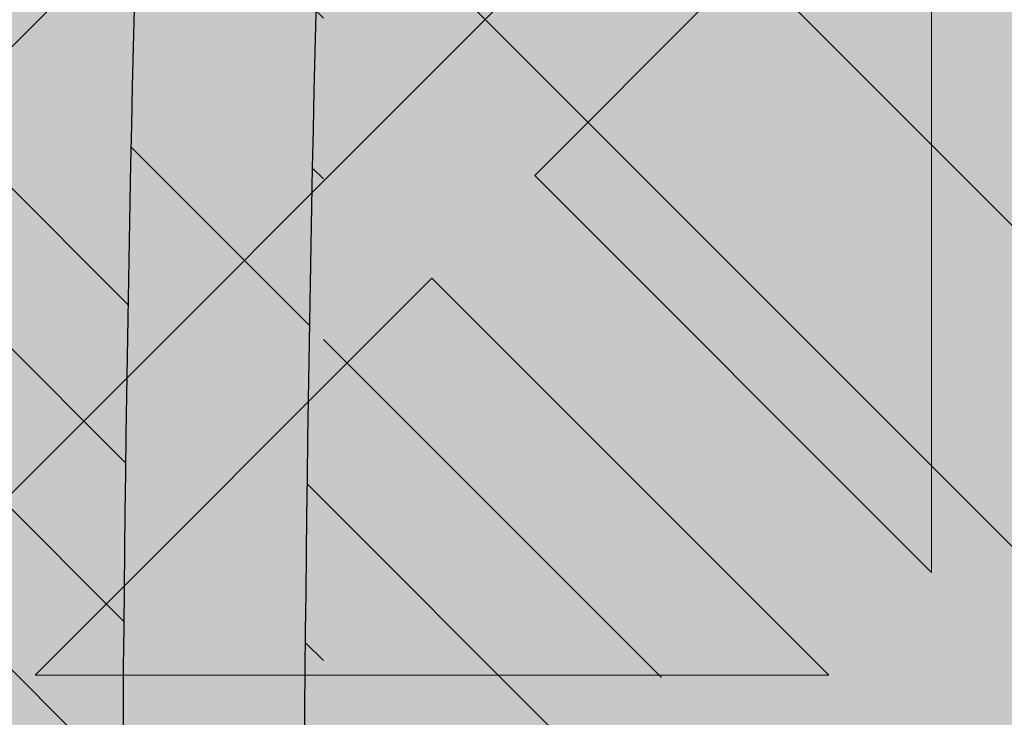
# Model space of a CAD drawing. Units: inches. Extents: x 844 to 2234, y 346 to 1084.
# Tile 80 of 93: x 2002.13 to 2003.858, y 703.938 to 705.162. Entities that reach past the tile are written whole.
import ezdxf

# ---------------------------------------------------------------- set-up
doc = ezdxf.new("R2010")
doc.units = ezdxf.units.IN
doc.header["$MEASUREMENT"] = 0
for name, color, linetype, lineweight in [('A-ANNO-DIMS', 2, 'Continuous', 18), ('furniture', 8, 'Continuous', 18), ('RA-AP-01$0$INT', 35, 'Continuous', 5)]:
    doc.layers.add(name, color=color, linetype=linetype, lineweight=lineweight)
doc.layers.add('RA-AP-01$0$FURN', color=3, linetype='Continuous')
doc.layers.add('RA-AP-01$0$WOOD', color=64, linetype='Continuous')
doc.styles.get("Standard").update_dxf_attribs({"font": 'arial.ttf'})
doc.dimstyles.get("Standard").update_dxf_attribs({"dimtxt": 6, "dimasz": 3, "dimexe": 0.18, "dimexo": 0.0625, "dimgap": 0.09, "dimtad": 0, "dimtih": 1, "dimtoh": 1, "dimdec": 1, "dimzin": 0, "dimdsep": 46, "dimlunit": 3, "dimtxsty": 'Standard', "dimblk": 'ARCHTICK', "dimcen": 0.09, "dimadec": 0, "dimazin": 0, "dimtfac": 1, "dimtdec": 1, "dimtofl": 0, "dimtmove": 0, "dimatfit": 3, "dimfxl": 1, "dimtolj": 1, "dimtzin": 0, "dimarcsym": 0})

# ---------------------------------------------------------------- blocks, each defined once
blk = doc.blocks.new('A$C18D01794')
at = {"layer": 'RA-AP-01$0$INT'}
h = blk.add_hatch(color=256, dxfattribs=at)
h.paths.add_polyline_path([(4.585917135068448, -7.856712009587804), (4.614201406330596, -7.856712009587056), (4.668846067270487, -7.802067348644738), (4.723490728212344, -7.856712009584164), (4.771774999457151, -7.856712009582887), (4.826419660396886, -7.80206734864072), (4.862780050090322, -7.838427738332541), (4.844495778842715, -7.856712009580965), (4.862780050090411, -7.856712009580482), (4.905206456960182, -7.814285602707865), (4.947632863832445, -7.856712009578238), (4.965917135079675, -7.856712009577755), (4.947632863831759, -7.838427738330656), (4.983993253523576, -7.802067348637219), (5.038637914464627, -7.856712009575829), (5.08692218571208, -7.856712009574554), (5.141566846649976, -7.802067348634224), (5.196211507589851, -7.856712009571666), (5.224495778822615, -7.856712009570916), (4.905206456953975, -7.537422687702283)])
h.paths.add_polyline_path([(4.895206456956031, -7.575706958950402), (4.895206456958921, -7.684996280828174), (4.840561796018589, -7.630351619890275)], flags=16)
h.paths.add_polyline_path([(4.915206456955638, -7.575706958949956), (4.969851117895509, -7.630351619887399), (4.915206456957609, -7.684996280827732)], flags=16)
h.paths.add_polyline_path([(4.826419660395175, -7.644493755514321), (4.881064321335613, -7.699138416452331), (4.771774999456703, -7.69913841645522)], flags=16)
h.paths.add_polyline_path([(4.983993253519558, -7.644493755510815), (5.038637914460456, -7.699138416449285), (4.929348592581548, -7.69913841645126)], flags=16)
h.paths.add_polyline_path([(4.881064321336025, -7.719138416452334), (4.826419660397532, -7.773783077393256), (4.771774999457062, -7.719138416455217)], flags=16)
h.paths.add_polyline_path([(4.929348592582019, -7.71913841645126), (5.038637914460982, -7.719138416449284), (4.983993253522945, -7.773783077389749)], flags=16)
h.paths.add_polyline_path([(4.895206456960191, -7.733280552075633), (4.895206456962115, -7.806001331460164), (4.876922185715016, -7.824285602708492), (4.840561796021581, -7.787925213016675)], flags=16)
h.paths.add_polyline_path([(4.915206456958487, -7.733280552075187), (4.969851117899527, -7.787925213013798), (4.933490728206909, -7.824285602708034), (4.9152064569598, -7.806001331461736)], flags=16)
h.paths.add_polyline_path([(4.757632863832376, -7.733280552079264), (4.812277524772842, -7.787925213017304), (4.757632863834348, -7.842569873958233)], flags=16)
h.paths.add_polyline_path([(4.737632863832376, -7.73328055207979), (4.737632863834348, -7.842569873958701), (4.682988202893906, -7.787925213020692)], flags=16)
h.paths.add_polyline_path([(5.05278005008503, -7.733280552072701), (5.052780050087917, -7.842569873951664), (4.998135389146995, -7.787925213013169)], flags=16)
h.paths.add_polyline_path([(5.072780050085024, -7.733280552072333), (5.127424711025931, -7.787925213010806), (5.072780050087916, -7.842569873951244)], flags=16)
h.paths.add_polyline_path([(4.935917135072783, -7.506712009583784), (5.255206456948811, -7.826001331459767), (5.255206456948932, -7.797717060211899), (5.200561796010279, -7.743072399273238), (5.255206456949403, -7.688427738334128), (5.25520645694961, -7.640143467086677), (5.200561796009787, -7.585498806146837), (5.236922185702417, -7.549138416454212), (5.255206456949919, -7.56742268770172), (5.255206456949998, -7.549138416454178), (5.212780050078687, -7.506712009583814), (5.25520645695036, -7.464285602712145), (5.255206456950438, -7.446001331464763), (5.236922185702424, -7.464285602712779), (5.200561796009796, -7.427925213020149), (5.255206456950753, -7.373280552079203), (5.25520645695096, -7.324996280834394), (5.200561796010322, -7.270351619893748), (5.255206456951428, -7.215706958952649), (5.255206456951547, -7.187422687705071)])
h.paths.add_polyline_path([(5.042988202883395, -7.42792521302065), (5.097632863823085, -7.373280552080975), (5.097632863822622, -7.482569873959883)], flags=16)
h.paths.add_polyline_path([(5.028846067259663, -7.442067348644384), (5.083490728198774, -7.496712009583504), (4.974201406321001, -7.496712009583035)], flags=16)
h.paths.add_polyline_path([(5.117632863823087, -7.37328055208089), (5.172277524762331, -7.42792521302015), (5.11763286382262, -7.482569873959851)], flags=16)
h.paths.add_polyline_path([(5.08349072819877, -7.516712009582191), (5.028846067259652, -7.571356670521302), (4.974201406320998, -7.516712009582638)], flags=16)
h.paths.add_polyline_path([(5.131774999446817, -7.35913841645716), (5.186419660386065, -7.413783077396415), (5.241064321325782, -7.359138416456712)], flags=17)
h.paths.add_polyline_path([(5.131774999446228, -7.496712009583703), (5.186419660386065, -7.442067348643883), (5.222780050079488, -7.478427738337313), (5.204495778832781, -7.496712009584014)], flags=16)
h.paths.add_polyline_path([(5.097632863822613, -7.530854145205813), (5.097632863823061, -7.640143467084723), (5.042988202883383, -7.585498806145032)], flags=16)
h.paths.add_polyline_path([(5.131774999446899, -7.339138416457162), (5.241064321325809, -7.339138416456712), (5.186419660386591, -7.284493755517479)], flags=17)
h.paths.add_polyline_path([(5.131774999446226, -7.516712009581999), (5.204495778830767, -7.516712009581702), (5.22278005007868, -7.534996280829206), (5.186419660386049, -7.571356670521828)], flags=16)
h.paths.add_polyline_path([(5.11763286382262, -7.530854145205852), (5.17227752476232, -7.585498806145562), (5.117632863823064, -7.64014346708481)], flags=16)
h.paths.add_polyline_path([(5.186419660386069, -7.599640941770585), (5.241064321325754, -7.654285602710281), (5.131774999446791, -7.654285602709814)], flags=16)
h.paths.add_polyline_path([(5.131774999446872, -7.674285602709813), (5.24106432132578, -7.674285602710282), (5.186419660386554, -7.728930263649504)], flags=16)
h.paths.add_polyline_path([(5.255206456951811, -7.126001331467467), (5.255206456951895, -7.106712009588038), (4.555206456956052, -7.106712009588038), (4.555206456956136, -7.12600133146746), (4.905206456953973, -7.476001331465289)])
h.paths.add_polyline_path([(4.983993253513404, -7.368930263651977), (4.92934859257295, -7.314285602713969), (5.03863791445186, -7.314285602711063)], flags=16)
h.paths.add_polyline_path([(4.969851117889988, -7.383072399276016), (4.915206456952556, -7.437717060215906), (4.915206456949648, -7.328427738338133)], flags=16)
h.paths.add_polyline_path([(4.929348592572535, -7.294285602713971), (4.983993253511019, -7.239640941773039), (5.038637914451496, -7.294285602711065)], flags=16)
h.paths.add_polyline_path([(5.052780050074912, -7.280143467087016), (4.998135389134438, -7.225498806148989), (5.052780050072919, -7.170854145208052)], flags=16)
h.paths.add_polyline_path([(5.07278005007491, -7.280143467086489), (5.072780050072918, -7.170854145207579), (5.127424711013374, -7.225498806145578)], flags=16)
h.paths.add_polyline_path([(4.89520645695295, -7.437717060216355), (4.840561796013067, -7.383072399278919), (4.895206456950961, -7.328427738338582)], flags=16)
h.paths.add_polyline_path([(4.915206456948365, -7.280143467090674), (4.915206456946434, -7.207422687704125), (4.933490728192729, -7.18913841645701), (4.969851117886972, -7.225498806149623)], flags=16)
h.paths.add_polyline_path([(4.881064321327021, -7.314285602715054), (4.82641966038902, -7.368930263655506), (4.771774999448108, -7.314285602717047)], flags=16)
h.paths.add_polyline_path([(4.895206456950073, -7.280143467091125), (4.840561796009022, -7.225498806152518), (4.876922185700835, -7.18913841645908), (4.895206456948749, -7.207422687706589)], flags=16)
h.paths.add_polyline_path([(4.983993253510392, -7.211356670525576), (4.947632863816944, -7.174996280833758), (4.965917135064043, -7.156712009585847), (5.038637914448995, -7.156712009584522)], flags=16)
h.paths.add_polyline_path([(4.881064321326543, -7.294285602715056), (4.771774999447578, -7.294285602717046), (4.826419660385607, -7.239640941776569)], flags=16)
h.paths.add_polyline_path([(4.905206456946447, -7.19913841645844), (4.862780050074785, -7.156712009587725), (4.947632863816685, -7.156712009586302)], flags=16)
h.paths.add_polyline_path([(5.14156684663679, -7.211356670521528), (5.086922185696452, -7.156712009583639), (5.196211507574223, -7.156712009581651)], flags=16)
h.paths.add_polyline_path([(4.8264196603837, -7.211356670529104), (4.771774999442643, -7.156712009590501), (4.8444957788276, -7.156712009588568), (4.862780050075511, -7.17499628083566)], flags=16)
h.paths.add_polyline_path([(4.812277524760289, -7.225498806153156), (4.757632863822258, -7.28014346709363), (4.757632863819352, -7.170854145214669)], flags=16)
h.paths.add_polyline_path([(4.73763286382226, -7.280143467093997), (4.682988202881349, -7.22549880615554), (4.737632863819352, -7.170854145215086)], flags=16)
h.paths.add_polyline_path([(4.723490728195188, -7.156712009591787), (4.668846067257299, -7.211356670532127), (4.614201406317417, -7.156712009594693)], flags=16)
h.paths.add_polyline_path([(4.597632863829262, -7.506712009583814), (4.555206456957951, -7.54913841645418), (4.555206456958029, -7.56742268770172), (4.573490728205535, -7.549138416454212), (4.609851117898167, -7.585498806146839), (4.555206456958338, -7.640143467086675), (4.555206456958546, -7.688427738334125), (4.60985111789767, -7.743072399273238), (4.555206456959015, -7.797717060211899), (4.555206456959138, -7.826001331459767), (4.874495778835167, -7.506712009583786), (4.5552064569564, -7.187422687705062), (4.555206456956523, -7.215706958952644), (4.609851117897629, -7.270351619893746), (4.555206456956988, -7.324996280834396), (4.555206456957198, -7.373280552079195), (4.609851117898153, -7.427925213020147), (4.573490728205528, -7.464285602712779), (4.555206456957507, -7.446001331464756), (4.555206456957585, -7.464285602712143)])
h.paths.add_polyline_path([(4.712780050085332, -7.482569873959882), (4.712780050084863, -7.373280552080972), (4.767424711024555, -7.42792521302065)], flags=16)
h.paths.add_polyline_path([(4.726922185709173, -7.496712009583504), (4.781566846648288, -7.442067348644384), (4.836211507586949, -7.496712009583033)], flags=16)
h.paths.add_polyline_path([(4.692780050085327, -7.482569873959851), (4.638135389145619, -7.427925213020149), (4.692780050084865, -7.373280552080892)], flags=16)
h.paths.add_polyline_path([(4.726922185709182, -7.516712009582191), (4.836211507586949, -7.51671200958264), (4.7815668466483, -7.571356670521304)], flags=16)
h.paths.add_polyline_path([(4.678637914461726, -7.496712009583706), (4.605917135075169, -7.496712009584014), (4.587632863828464, -7.478427738337311), (4.623993253521887, -7.442067348643881)], flags=16)
h.paths.add_polyline_path([(4.712780050085336, -7.530854145205816), (4.767424711024568, -7.585498806145034), (4.71278005008489, -7.640143467084724)], flags=16)
h.paths.add_polyline_path([(4.678637914461726, -7.516712009582001), (4.623993253521899, -7.571356670521829), (4.587632863829271, -7.534996280829206), (4.605917135077185, -7.5167120095817)], flags=16)
h.paths.add_polyline_path([(4.692780050085336, -7.530854145205848), (4.692780050084889, -7.64014346708481), (4.638135389145632, -7.585498806145562)], flags=16)
h.paths.add_polyline_path([(4.623993253521885, -7.413783077396415), (4.678637914461131, -7.359138416457161), (4.56934859258217, -7.359138416456712)], flags=17)
h.paths.add_polyline_path([(4.623993253521901, -7.599640941770568), (4.678637914461158, -7.654285602709814), (4.569348592582195, -7.654285602710281)], flags=16)
h.paths.add_polyline_path([(4.678637914461051, -7.339138416457162), (4.623993253521361, -7.284493755517479), (4.569348592582143, -7.339138416456712)], flags=17)
h.paths.add_polyline_path([(4.678637914461076, -7.674285602709813), (4.623993253521399, -7.728930263649504), (4.569348592582167, -7.674285602710281)], flags=16)
h = blk.add_hatch(color=256, dxfattribs=at)
h.paths.add_polyline_path([(4.905206456954232, -7.537422687702028), (4.874495778835232, -7.506712009583718), (4.555206456959138, -7.826001331459766), (4.555206456959269, -7.856712009588616), (4.585917135068449, -7.856712009587804)])
h.paths.add_polyline_path([(4.935917135072152, -7.506712009583152), (4.905206456953497, -7.537422687701806), (5.224495778822614, -7.856712009570917), (5.255206456948681, -7.856712009570104), (5.255206456948813, -7.826001331459768)])
h.paths.add_polyline_path([(5.255206456951549, -7.18742268770507), (5.255206456951813, -7.126001331467461), (4.905206456953563, -7.476001331465701), (4.935917135072559, -7.506712009584006)])
h.paths.add_polyline_path([(4.874495778835167, -7.506712009583785), (4.905206456953818, -7.476001331465132), (4.555206456956135, -7.126001331467458), (4.555206456956399, -7.187422687705064)])
h = blk.add_hatch(color=256, dxfattribs=at)
h.paths.add_polyline_path([(4.89520645695096, -7.328427738338579), (4.840561796013068, -7.383072399278921), (4.89520645695295, -7.437717060216353)])
h.paths.add_polyline_path([(4.915206456952557, -7.437717060215907), (4.969851117889986, -7.383072399276024), (4.915206456949648, -7.328427738338133)])
h.paths.add_polyline_path([(4.929348592572952, -7.31428560271397), (4.983993253513403, -7.368930263651974), (5.038637914451863, -7.314285602711064)])
h.paths.add_polyline_path([(5.038637914451498, -7.294285602711065), (4.983993253511018, -7.239640941773039), (4.929348592572535, -7.294285602713969)])
h.paths.add_polyline_path([(4.969851117886971, -7.225498806149624), (4.93349072819273, -7.189138416457011), (4.915206456946433, -7.207422687704124), (4.915206456948367, -7.280143467090678)])
h.paths.add_polyline_path([(4.965917135064045, -7.156712009585847), (4.947632863816945, -7.17499628083376), (4.983993253510389, -7.211356670525573), (5.038637914448995, -7.156712009584522)])
h.paths.add_polyline_path([(4.998135389134439, -7.22549880614899), (5.05278005007491, -7.280143467087016), (5.052780050072921, -7.170854145208054)])
h.paths.add_polyline_path([(5.072780050074911, -7.28014346708649), (5.127424711013374, -7.225498806145579), (5.072780050072921, -7.170854145207581)])
h.paths.add_polyline_path([(5.196211507574225, -7.156712009581651), (5.08692218569645, -7.156712009583639), (5.141566846636789, -7.211356670521529)])
h.paths.add_polyline_path([(4.862780050074782, -7.156712009587723), (4.90520645694645, -7.199138416458444), (4.94763286381669, -7.156712009586302)])
h.paths.add_polyline_path([(4.895206456950073, -7.280143467091126), (4.895206456948746, -7.207422687706587), (4.876922185700836, -7.189138416459078), (4.840561796009025, -7.225498806152521)])
h.paths.add_polyline_path([(4.826419660385605, -7.239640941776569), (4.771774999447577, -7.294285602717049), (4.881064321326541, -7.294285602715055)])
h.paths.add_polyline_path([(4.771774999448108, -7.314285602717046), (4.82641966038902, -7.368930263655505), (4.88106432132702, -7.314285602715054)])
h.paths.add_polyline_path([(4.757632863822258, -7.280143467093631), (4.812277524760285, -7.225498806153153), (4.757632863819352, -7.170854145214668)])
h.paths.add_polyline_path([(4.862780050075512, -7.17499628083566), (4.844495778827599, -7.156712009588567), (4.771774999442647, -7.156712009590504), (4.8264196603837, -7.211356670529104)])
h.paths.add_polyline_path([(4.682988202881349, -7.225498806155537), (4.737632863822258, -7.280143467093997), (4.737632863819352, -7.170854145215087)])
h.paths.add_polyline_path([(4.723490728195189, -7.156712009591783), (4.614201406317418, -7.156712009594692), (4.668846067257298, -7.211356670532127)])
for p, q in [((4.905206456953975, -7.476001331465289), (5.255206456951811, -7.126001331467465)), ((4.935917135072783, -7.506712009583784), (5.255206456951548, -7.187422687705069)), ((4.929348592572952, -7.314285602713971), (4.983993253513403, -7.368930263651975)), ((5.038637914451862, -7.314285602711064), (4.929348592572952, -7.314285602713971)), ((4.983993253513404, -7.368930263651973), (5.038637914451862, -7.314285602711064)), ((4.915206456949651, -7.328427738338136), (4.969851117889986, -7.383072399276024)), ((4.915206456949648, -7.328427738338135), (4.915206456952556, -7.437717060215906)), ((4.915206456952556, -7.437717060215906), (4.969851117889986, -7.383072399276024))]:
    blk.add_line(p, q, dxfattribs=at)
blk = doc.blocks.new('A$C32926AE1')
at = {"layer": 'RA-AP-01$0$FURN'}
h = blk.add_hatch(dxfattribs=at)
h.set_pattern_fill('ANSI31', color=256, scale=0.1, style=0)
h.set_pattern_definition([(45, (0, 0), (-0.0088388347648318, 0.0088388347648318), [])])
edge = h.paths.add_edge_path(flags=16)
edge.add_arc((4.904771284329206, 4.246793130718756), 0.2603971832811541, 75.22398030683196, 104.7760196931204)
edge.add_arc((4.904771284329206, 4.246793130718756), 0.2603971832811541, 75.223980306832, 104.77601969312039, ccw=False)
edge = h.paths.add_edge_path(flags=16)
edge.add_arc((4.904771284329206, 4.067062675376612), 0.2603971832811541, 255.2239803068796, 284.776019693168)
edge.add_arc((4.904771284329206, 4.067062675376612), 0.2603971832811541, 255.22398030687958, 284.77601969316805, ccw=False)
edge = h.paths.add_edge_path(flags=0)
edge.add_arc((4.904771284329206, 4.067062675376612), 0.2603971832811541, 255.2239803068796, 284.776019693168)
edge.add_arc((4.904771284329206, 4.067062675376612), 0.2603971832811541, 255.22398030687958, 284.77601969316805, ccw=False)
edge = h.paths.add_edge_path(flags=0)
edge.add_arc((4.904771284329206, 4.067062675376612), 0.2603971832811541, 255.2239803068796, 284.776019693168)
edge.add_arc((4.904771284329206, 4.067062675376612), 0.2603971832811541, 255.22398030687958, 284.77601969316805, ccw=False)
edge = h.paths.add_edge_path()
edge.add_arc((4.604388392048174, 4.588829985554312), 0.1599999999999918, 342.3781640246255, 354.4317409793762)
edge.add_arc((5.090145208887507, 4.43216705527679), 0.3503971832811637, 162.0091218307731, 180.3186872093483)
edge.add_arc((5.205154176610243, 4.588829985554953), 0.1599999999999917, 185.5682590208461, 197.6218359767349)
edge.add_arc((4.904771284329229, 4.246793130718735), 0.3503971832811761, 72.00912183053516, 107.9908781690354)
edge.add_arc((9.535952835716557, 4.28682295566602), 4.798342501046485, 178.2875002453811, 181.5576802719453)
edge.add_arc((4.719397359771122, 4.43216705527679), 0.3503971832811637, 359.6813127906516, 377.9908781692269)
edge.add_arc((9.535967292294904, 4.286822350292874), 4.778371420254705, 178.2965938931842, 181.5667745797229)
edge.add_arc((4.719397359771122, 4.43216705527679), 0.3303971832811637, 359.6813127906516, 377.9908781692269)
edge.add_arc((0.2735752763637294, 4.286822350292874), 4.7783714202547, 358.4332254202771, 361.7034061068158)
edge.add_arc((5.061434214606998, 4.732549947558029), 0.1600000000000254, 252.3781640250584, 264.4317409792362)
edge.add_arc((4.748108354051257, 4.732549947558012), 0.1600000000000541, 275.5682590208426, 287.6218359759532)
edge.add_arc((4.604388392048115, 4.588829985554317), 0.1800000000000505, 342.3567572500182, 349.3735009646207)
edge.add_arc((5.205154176610254, 4.588829985554976), 0.1800000000000069, 190.6264990356027, 197.6432427513933)
edge.add_arc((5.061434214607106, 4.732549947558013), 0.1800000000000424, 252.3567572496606, 259.3735009644582)
edge.add_arc((4.904771284329208, 4.246793130718737), 0.3303971832811676, 71.99844483668534, 108.0015551637021)
edge.add_arc((4.748108354051414, 4.732549947558045), 0.1800000000000547, 280.6264990355479, 287.6432427495938)
edge.add_arc((5.090145208887514, 4.432167055276789), 0.2803971832811691, 162.8706300666893, 180.816523289902)
edge.add_arc((4.719397359771136, 4.432167055276689), 0.2803971832811534, 359.183476710103, 377.1293699333214)
edge.add_arc((4.904771284329222, 4.246793130718737), 0.2803971832811769, 72.87063006672916, 107.1293699332334)
edge.add_arc((5.090145208887522, 4.432167055276788), 0.2603971832811776, 165.2239803068007, 180.9953123810312)
edge.add_arc((4.719397359771141, 4.432167055276699), 0.2603971832811458, 359.0046876189768, 374.7760196932087)
edge.add_arc((5.090145208887507, 4.43216705527679), 0.3303971832811637, 162.0091218307731, 180.3186872093483)
edge.add_arc((9.53595427642584, 4.285015535491528), 4.728345371032053, 178.265043920078, 181.5679956281801)
edge.add_arc((0.2735882922327999, 4.285015535491582), 4.728345371032045, 358.4320043718193, 361.7349560799204)
edge.add_arc((9.535953591267507, 4.284458026472751), 4.708343996644348, 178.2573054306777, 181.5704995759608)
edge.add_arc((0.273588977391114, 4.284458026472785), 4.708343996644358, 358.4295004240388, 361.7426945693213)
edge.add_arc((0.2735889773911131, 4.029397779622582), 4.708343996644359, 358.2573054306787, 361.5704995759613)
edge.add_arc((9.535953591267518, 4.029397779622618), 4.708343996644359, 178.4295004240391, 181.7426945693223)
edge.add_arc((0.2735882922327901, 4.028840270603786), 4.728345371032054, 358.2650439200796, 361.5679956281808)
edge.add_arc((9.53595427642584, 4.028840270603841), 4.728345371032054, 178.4320043718199, 181.7349560799219)
edge.add_arc((0.2735752763637302, 4.027033455802493), 4.778371420254699, 358.2965938931842, 361.5667745797229)
edge.add_arc((4.719397359771122, 3.881688750818578), 0.3303971832811637, 342.0091218307731, 360.3186872093484)
edge.add_arc((5.090145208887507, 3.881688750818578), 0.3303971832811637, 179.6813127906516, 197.9908781692269)
edge.add_arc((9.535967292294904, 4.027033455802493), 4.778371420254705, 178.433225420277, 181.7034061068158)
edge.add_arc((4.719397359771122, 3.881688750818578), 0.3503971832811637, 342.0091218307731, 360.3186872093484)
edge.add_arc((9.53595283571655, 4.027032850429349), 4.79834250104648, 178.4423197280546, 181.7124997546188)
edge.add_arc((4.719397359771141, 3.881688750818669), 0.2603971832811458, 345.2239803067913, 360.9953123810232)
edge.add_arc((5.090145208887522, 3.88168875081858), 0.2603971832811776, 179.0046876189687, 194.7760196931993)
edge.add_arc((4.904771284329222, 4.067062675376631), 0.2803971832811769, 252.8706300667665, 287.1293699332708)
edge.add_arc((4.719397359771136, 3.881688750818678), 0.2803971832811534, 342.8706300666787, 360.8165232898969)
edge.add_arc((5.090145208887514, 3.881688750818579), 0.2803971832811691, 179.183476710098, 197.1293699333106)
edge.add_arc((4.748108354051414, 3.581305858537323), 0.1800000000000547, 72.3567572504062, 79.37350096445199)
edge.add_arc((4.904771284329208, 4.067062675376631), 0.3303971832811676, 251.9984448362979, 288.0015551633146)
edge.add_arc((5.061434214607106, 3.581305858537355), 0.1800000000000424, 100.6264990355418, 107.6432427503394)
edge.add_arc((5.205154176610254, 3.725025820540392), 0.1800000000000069, 162.3567572486066, 169.3735009643972)
edge.add_arc((4.604388392048115, 3.725025820541051), 0.1800000000000505, 10.62649903537925, 17.64324274998182)
edge.add_arc((4.748108354051257, 3.581305858537356), 0.1600000000000541, 72.37816402404681, 84.43174097915735)
edge.add_arc((4.904771284329229, 4.067062675376632), 0.3503971832811761, 252.0091218309645, 287.9908781694648)
edge.add_arc((5.061434214606998, 3.581305858537339), 0.1600000000000254, 95.56825902076373, 107.6218359749416)
edge.add_arc((5.205154176610243, 3.725025820540414), 0.1599999999999917, 162.3781640232651, 174.4317409791539)
edge.add_arc((5.090145208887507, 3.881688750818578), 0.3503971832811637, 179.6813127906516, 197.9908781692269)
edge.add_arc((4.604388392048174, 3.725025820541056), 0.1599999999999918, 5.568259020623824, 17.62183597537444)
edge.add_arc((0.2735897329420762, 4.28682295566602), 4.798342501046482, 358.4423197280547, 361.7124997546188)
edge.add_arc((0.2735897329420691, 4.027032850429348), 4.798342501046489, 358.2875002453812, 361.5576802719453)
at = {"layer": 'RA-AP-01$0$WOOD'}
h = blk.add_hatch(color=256, dxfattribs=at)
h.dxf.hatch_style = 1
h.paths.add_polyline_path([(5.157430609644524, 4.573483066760929, -0.1009492694046607), (5.155401577623758, 4.593365984175333, -0.1842662638101597), (5.172249623284174, 4.638795604568598, 0.2056608120311276), (5.179560981299304, 4.661316324430096, 0.3614336704623542), (5.134352340494423, 4.706524965234944, 0.2056608120311297), (5.111831620632933, 4.699213607219793, -0.1842662638101113), (5.066402000239693, 4.682365561559342, -0.1055311479399994), (5.045656153913092, 4.68467289944697, 0.1567636581983829), (4.763886414745334, 4.684672899446966, -0.1055311479399895), (4.743140568418733, 4.68236556155934, -0.1842662638100833), (4.6977109480255, 4.69921360721979, 0.2056608120302612), (4.675190228164109, 4.706524965234949, 0.3614336704708441), (4.629981587358889, 4.66131632442871, 0.2056608120245944), (4.637292945374126, 4.638795604567974, -0.1842662638101024), (4.654140991034615, 4.59336598417475, -0.1009492694055169), (4.652111959013835, 4.573483066760181, 0.021410119221476), (4.629748025606143, 4.156712009541676, 0.0214101192214795), (4.652111959013809, 3.739940952323101, -0.1009492694059586), (4.654140991034615, 3.720058034908448, -0.1842662638100975), (4.637292945374126, 3.674628414515226, 0.2056608120245705), (4.629981587358889, 3.652107694654492, 0.3614336704708879), (4.675190228164113, 3.606899053848249, 0.2056608120302384), (4.697710948025501, 3.614210411863408, -0.1842662638100995), (4.743140568418738, 3.63105845752386, -0.1055311479402541), (4.763886414745388, 3.628751119636215, 0.1567636581983776), (5.045656153913137, 3.628751119636244, -0.1055311479397538), (5.066402000239692, 3.631058457523857, -0.1842662638101067), (5.111831620632931, 3.614210411863407, 0.2056608120310924), (5.134352340494417, 3.606899053848256, 0.3614336704624001), (5.179560981299307, 3.652107694653103, 0.2056608120311314), (5.172249623284175, 3.6746284145146, -0.1842662638101402), (5.155401577623758, 3.72005803490786, -0.1009492694051366), (5.15743060964455, 3.739940952322354, 0.0214101192215073), (5.179794543052287, 4.156712009541468, 0.0214101192215252)])
h.paths.add_polyline_path([(4.639748609479751, 4.156712009541513, 0.0213537860821624), (4.661970494867118, 3.741887061152232, -0.094075836301374), (4.664143710413708, 3.7196126951003, -0.1824818158568985), (4.644813765429836, 3.668037719127816, 0.2056608120245319), (4.639939526753007, 3.653023905887301, 0.3614336704710246), (4.676106439397173, 3.616856993242342, 0.2056608120302234), (4.691120252638095, 3.621731231919122, -0.1824818158602558), (4.742695228611606, 3.641061176902986, -0.1029891339458722), (4.766991894714349, 3.638256818950944, 0.156709409989566), (5.042550673941472, 3.638256818950105, -0.102989133958497), (5.066847340047078, 3.641061176902949, -0.1824818158594995), (5.118422316020358, 3.621731231919103, 0.2056608120311416), (5.133436129261316, 3.616856993242346, 0.3614336704621468), (5.169603041905217, 3.653023905886178, 0.2056608120310986), (5.164728803228477, 3.668037719127177, -0.1824818158565612), (5.145398858244737, 3.719612695099578, -0.0940758363009313), (5.147572073791232, 3.741887061151398, 0.0213537860822023), (5.169793959178681, 4.156712009541451, 0.0213537860822226), (5.147572073791203, 4.571536957931898, -0.0940758363005034), (5.145398858244737, 4.59381132398362, -0.1824818158565587), (5.164728803228476, 4.645386299956021, 0.2056608120311045), (5.169603041905216, 4.66040011319702, 0.3614336704621845), (5.133436129261313, 4.696567025840856, 0.2056608120310773), (5.118422316020359, 4.691692787164098, -0.182481815859508), (5.066847340047078, 4.67236284218025, -0.1029891339584606), (5.04255067394148, 4.675167200133092, 0.156709409989566), (4.766991894714357, 4.675167200132257, -0.1029891339458842), (4.742695228611611, 4.672362842180213, -0.1824818158602725), (4.691120252638095, 4.691692787164077, 0.2056608120302152), (4.676106439397174, 4.696567025840858, 0.3614336704710363), (4.639939526753005, 4.660400113195899, 0.2056608120245495), (4.644813765429837, 4.645386299955384, -0.1824818158568934), (4.664143710413708, 4.593811323982902, -0.0940758363009187), (4.661970494867149, 4.571536957931074, 0.021353786082177)], flags=16)
h.paths.add_polyline_path([(5.129794543052235, 4.432167055276933, -0.0141661062790638), (5.130152669293814, 4.156927903047693, -0.0141661062790647), (5.129794543052234, 3.881688750818433, -0.0785247771143638), (5.10979738006795, 3.755143611847103, 0.0945969212073497), (5.105408519571111, 3.717898134952927, 0.1043170707844957), (5.116074640131521, 3.670385395016088, 0.1043170707864965), (5.068561900193738, 3.681051515576561, 0.09459692119553), (5.031316423304057, 3.676662655080835, -0.1580239521427272), (4.778226145355827, 3.676662655080367, 0.0945969211986668), (4.740980668464973, 3.681051515576592, 0.1043170707882822), (4.693467928526415, 3.670385395015844, 0.1043170707867916), (4.704134049087309, 3.717898134953662, 0.0945969211972894), (4.69974518859162, 3.755143611844042, -0.0785247771163196), (4.679748025606343, 3.881688750818406, -0.0141661062790663), (4.679389899364763, 4.156927903047693, -0.0141661062790672), (4.679748025606343, 4.432167055276998, -0.0785247771163064), (4.699745188591625, 4.55871219425134, 0.094596921197333), (4.704134049087308, 4.595957671141738, 0.1043170707867205), (4.693467928526416, 4.643470411079523, 0.1043170707882628), (4.740980668464965, 4.632804290518776, 0.0945969211988114), (4.778226145355874, 4.637193151015016, -0.158023952142669), (5.031316423304015, 4.637193151014546, 0.0945969211956361), (5.068561900193736, 4.632804290518806, 0.1043170707864979), (5.11607464013152, 4.643470411079278, 0.1043170707844617), (5.105408519571112, 4.595957671142455, 0.0945969212074597), (5.109797380067959, 4.558712194248236, -0.0785247771143467)], flags=0)
h.paths.add_polyline_path([(5.119794532311105, 4.432259799204851, -0.0142000800617244), (5.120156169157484, 4.156927903047701, -0.0142000800617277), (5.119794532311105, 3.881596006890482, -0.0784894509520253), (5.100273383573699, 3.758192358677797, 0.0940138827242913), (5.095413455884425, 3.717477693979438, 0.0606271852308753), (5.099615656341024, 3.686844378806616, 0.0606271852322524), (5.068982341167493, 3.691046579263239, 0.0940138827010453), (5.028267676478798, 3.686186651576848, -0.1580706864508061), (4.781274892180912, 3.686186651576435, 0.0940138827026903), (4.740560227491556, 3.691046579263279, 0.0606271852339895), (4.709926912317155, 3.686844378806508, 0.0606271852329405), (4.714129112773991, 3.717477693980356, 0.094013882701304), (4.709269185087677, 3.758192358669163, -0.0784894509577193), (4.689748036347473, 3.881596006890469, -0.014200080061729), (4.689386399501094, 4.156927903047709, -0.0142000800617217), (4.689748036347473, 4.432259799204808, -0.078489450957724), (4.709269185087651, 4.555663447426125, 0.0940138827014585), (4.714129112773992, 4.596378112114996, 0.0606271852329731), (4.709926912317154, 4.62701142728886, 0.0606271852340196), (4.74056022749157, 4.622809226832087, 0.0940138827024997), (4.781274892180847, 4.627669154518912, -0.1580706864508359), (5.028267676478777, 4.627669154518526, 0.0940138827010946), (5.068982341167492, 4.622809226832129, 0.060627185232254), (5.099615656341024, 4.627011427288751, 0.0606271852308727), (5.095413455884425, 4.59637811211593, 0.0940138827241088), (5.100273383573675, 4.555663447417647, -0.0784894509520978)], flags=0)
h.paths.add_polyline_path([(5.06978912287499, 4.430218106756144, -0.014241683694547), (5.070173729147532, 4.156927903047672, -0.0142416836945458), (5.06978912287499, 3.883637699339223, -0.0800609523125196), (5.052662118612511, 3.773463122773442, 0.0526421978001116), (5.04590916754064, 3.740550867606997, 0.0526421977992423), (5.012996912374707, 3.73379791653534, -0.1583028414718258), (4.796545656286308, 3.73379791653451, 0.0526421978034211), (4.763633401117837, 3.740550867607021, 0.0526421978018622), (4.756880450045755, 3.773463122774558, -0.0800609523117106), (4.739753445783639, 3.883637699339268, -0.0142416836945435), (4.739368839511098, 4.156927903047671, -0.0142416836945477), (4.739753445783639, 4.430218106756155, -0.0800609523116345), (4.75688045004574, 4.540392683320762, 0.052642197801941), (4.763633401117837, 4.573304938488346, 0.0526421978035071), (4.796545656286361, 4.580057889560873, -0.1583028414717561), (5.012996912374669, 4.580057889560039, 0.0526421977993048), (5.04590916754064, 4.57330493848837, 0.0526421978002057), (5.052662118612529, 4.540392683321868, -0.080060952312477)], flags=0)
h.paths.add_polyline_path([(5.049789715110557, 4.43038092723357, -0.0143097550741839), (5.05018085590259, 4.156927903047715, -0.0143097550741854), (5.049789715110558, 3.883474878861827, -0.0800685599149176), (5.03362098255317, 3.779581877367999, 0.0306258898956367), (5.028241146483733, 3.758218888663947, 0.0306258898977031), (5.006878157778253, 3.75283905259408, -0.1583983521624096), (4.802664410878162, 3.752839052594731, 0.0306258898946014), (4.781301422174808, 3.758218888663924, 0.0306258898967912), (4.775921586105202, 3.779581877368794, -0.080068559914251), (4.759752853548071, 3.883474878861786, -0.0143097550741854), (4.759361712756037, 4.156927903047671, -0.0143097550741854), (4.759752853548071, 4.430380927233557, -0.0800685599142479), (4.775921586105193, 4.534273928726546, 0.0306258898968306), (4.781301422174808, 4.555636917431444, 0.0306258898945754), (4.802664410878143, 4.561016753500631, -0.1583983521624168), (5.006878157778244, 4.561016753501291, 0.0306258898977177), (5.028241146483733, 4.555636917431421, 0.0306258898958182), (5.03362098255321, 4.534273928727244, -0.080068559914796)], flags=0)
h.paths.add_polyline_path([(4.999766070382627, 4.428171244713864, -0.0143443147609634), (5.000198441819402, 4.156927903047689, -0.0143443147609612), (4.999766070382627, 3.885684561381556, -0.0784641635803329), (4.987356730658798, 3.799103304488872, -0.1506053783831347), (4.822185837999821, 3.79910330448882, -0.0784641635803318), (4.809776498276007, 3.885684561381509, -0.014344314760963), (4.809344126839227, 4.156927903047677, -0.0143443147609645), (4.809776498276007, 4.428171244713873, -0.0784641635803192), (4.822185837999822, 4.514752501606549, -0.1506053783831338), (4.987356730658798, 4.514752501606494, -0.078464163580285)], flags=0)
h.paths.add_polyline_path([(4.979755254238824, 4.42764379880488, -0.0143772539198268), (4.980205517789977, 4.156927903047693, -0.0143772539198275), (4.979755254238824, 3.886212007290489, -0.0689242507424422), (4.971183264704897, 3.815276770442801, -0.1296645318904179), (4.838359303953726, 3.815276770442746, -0.0689242507424186), (4.829787314419809, 3.886212007290419, -0.0143772539198292), (4.829337050868653, 4.156927903047653, -0.0143772539198325), (4.829787314419809, 4.427643798804946, -0.0689242507424211), (4.838359303953725, 4.498579035652621, -0.1296645318904187), (4.971183264704897, 4.498579035652565, -0.0689242507424401)], flags=0)
h = blk.add_hatch(color=256, dxfattribs=at)
h.dxf.hatch_style = 1
h.paths.add_polyline_path([(5.145398858244737, 4.59381132398362, -0.1824818158565616), (5.164728803228476, 4.645386299956021, 0.2056608120311045), (5.169603041905216, 4.66040011319702, 0.3614336704621845), (5.133436129261313, 4.696567025840856, 0.2056608120310773), (5.118422316020359, 4.691692787164098, -0.182481815859508), (5.066847340047078, 4.67236284218025, -0.1029891339584606), (5.04255067394148, 4.675167200133092, 0.156709409989566), (4.766991894714357, 4.675167200132257, -0.1029891339458842), (4.742695228611611, 4.672362842180213, -0.1824818158602725), (4.691120252638095, 4.691692787164077, 0.2056608120302152), (4.676106439397174, 4.696567025840858, 0.3614336704710363), (4.639939526753005, 4.660400113195899, 0.2056608120245495), (4.644813765429837, 4.645386299955384, -0.1824818158568934), (4.664143710413708, 4.593811323982902, -0.0940758363009187), (4.661970494867149, 4.571536957931074, 0.0213537860821772), (4.639748609479751, 4.156712009541507, 0.0213537860821625), (4.661970494867119, 3.741887061152226, -0.0940758363013071), (4.664143710413708, 3.719612695100309, -0.1824818158569294), (4.644813765429836, 3.668037719127816, 0.2056608120245319), (4.639939526753007, 3.653023905887301, 0.3614336704710246), (4.676106439397173, 3.616856993242342, 0.2056608120302234), (4.691120252638095, 3.621731231919122, -0.1824818158602558), (4.742695228611606, 3.641061176902986, -0.1029891339458722), (4.766991894714349, 3.638256818950944, 0.156709409989566), (5.042550673941472, 3.638256818950105, -0.102989133958497), (5.066847340047078, 3.641061176902949, -0.1824818158594995), (5.118422316020358, 3.621731231919103, 0.2056608120311416), (5.133436129261316, 3.616856993242346, 0.3614336704621468), (5.169603041905217, 3.653023905886178, 0.2056608120310986), (5.164728803228477, 3.668037719127177, -0.1824818158565612), (5.145398858244737, 3.719612695099578, -0.0940758363009313), (5.147572073791232, 3.741887061151398, 0.0213537860822023), (5.169793959178681, 4.156712009541451, 0.0213537860822226), (5.147572073791203, 4.571536957931898, -0.0940758363004996)])
h.paths.add_polyline_path([(5.109797380067958, 4.55871219424824, -0.0785247771143472), (5.129794543052234, 4.432167055276936, -0.0141661062790644), (5.130152669293814, 4.156927903047685, -0.014166106279066), (5.129794543052234, 3.881688750818401, -0.0785247771143517), (5.109797380067946, 3.755143611847092, 0.0945969212073132), (5.105408519571111, 3.717898134952929, 0.1043170707844995), (5.116074640131521, 3.670385395016088, 0.1043170707864965), (5.068561900193738, 3.681051515576561, 0.09459692119553), (5.031316423304057, 3.676662655080835, -0.1580239521427272), (4.778226145355827, 3.676662655080367, 0.0945969211986668), (4.740980668464973, 3.681051515576592, 0.1043170707882822), (4.693467928526415, 3.670385395015844, 0.1043170707867916), (4.704134049087309, 3.717898134953662, 0.0945969211972894), (4.69974518859162, 3.755143611844042, -0.0785247771163196), (4.679748025606343, 3.881688750818406, -0.0141661062790663), (4.679389899364763, 4.156927903047693, -0.0141661062790672), (4.679748025606343, 4.432167055276998, -0.0785247771163064), (4.699745188591625, 4.55871219425134, 0.094596921197333), (4.704134049087308, 4.595957671141738, 0.1043170707867205), (4.693467928526416, 4.643470411079523, 0.1043170707882628), (4.740980668464965, 4.632804290518776, 0.0945969211988114), (4.778226145355874, 4.637193151015016, -0.158023952142669), (5.031316423304015, 4.637193151014546, 0.0945969211956361), (5.068561900193736, 4.632804290518806, 0.1043170707864979), (5.11607464013152, 4.643470411079278, 0.1043170707844617), (5.105408519571112, 4.595957671142455, 0.0945969212074504)], flags=16)
h.paths.add_polyline_path([(5.100273383573655, 4.55566344741771, -0.0784894509521388), (5.119794532311105, 4.432259799204852, -0.0142000800617252), (5.120156169157484, 4.156927903047686, -0.014200080061726), (5.119794532311105, 3.881596006890502, -0.0784894509520446), (5.100273383573696, 3.758192358677786, 0.0940138827242721), (5.095413455884425, 3.717477693979436, 0.0606271852308692), (5.099615656341024, 3.686844378806616, 0.0606271852322522), (5.068982341167493, 3.691046579263239, 0.0940138827010453), (5.028267676478798, 3.686186651576848, -0.1580706864508061), (4.781274892180912, 3.686186651576435, 0.0940138827026903), (4.740560227491556, 3.691046579263279, 0.0606271852339895), (4.709926912317155, 3.686844378806508, 0.0606271852329405), (4.714129112773991, 3.717477693980356, 0.094013882701304), (4.709269185087677, 3.758192358669163, -0.0784894509577193), (4.689748036347473, 3.881596006890469, -0.014200080061729), (4.689386399501094, 4.156927903047709, -0.0142000800617217), (4.689748036347473, 4.432259799204808, -0.078489450957724), (4.709269185087651, 4.555663447426125, 0.0940138827014585), (4.714129112773992, 4.596378112114996, 0.0606271852329731), (4.709926912317154, 4.62701142728886, 0.0606271852340196), (4.74056022749157, 4.622809226832087, 0.0940138827024997), (4.781274892180847, 4.627669154518912, -0.1580706864508359), (5.028267676478777, 4.627669154518526, 0.0940138827010946), (5.068982341167492, 4.622809226832129, 0.060627185232254), (5.099615656341024, 4.627011427288751, 0.0606271852308727), (5.095413455884425, 4.59637811211593, 0.094013882723957)], flags=0)
h.paths.add_polyline_path([(5.04590916754064, 4.57330493848837, 0.0526421978002057), (5.052662118612529, 4.540392683321868, -0.0800609523124783), (5.06978912287499, 4.430218106756142, -0.0142416836945469), (5.070173729147532, 4.156927903047672, -0.0142416836945458), (5.06978912287499, 3.883637699339223, -0.0800609523125196), (5.052662118612511, 3.773463122773442, 0.0526421978001116), (5.04590916754064, 3.740550867606997, 0.0526421977992423), (5.012996912374707, 3.73379791653534, -0.1583028414718258), (4.796545656286308, 3.73379791653451, 0.0526421978034211), (4.763633401117837, 3.740550867607021, 0.0526421978018622), (4.756880450045755, 3.773463122774558, -0.0800609523117106), (4.739753445783639, 3.883637699339268, -0.0142416836945435), (4.739368839511098, 4.156927903047671, -0.0142416836945477), (4.739753445783639, 4.430218106756155, -0.0800609523116345), (4.75688045004574, 4.540392683320762, 0.052642197801941), (4.763633401117837, 4.573304938488346, 0.0526421978035071), (4.796545656286361, 4.580057889560873, -0.1583028414717561), (5.012996912374669, 4.580057889560039, 0.0526421977993048)], flags=0)
h.paths.add_polyline_path([(5.028241146483733, 4.555636917431422, 0.0306258898956949), (5.033620982553182, 4.534273928727329, -0.0800685599148649), (5.049789715110557, 4.430380927233569, -0.0143097550741839), (5.05018085590259, 4.156927903047715, -0.0143097550741854), (5.049789715110558, 3.883474878861827, -0.0800685599149176), (5.03362098255317, 3.779581877367999, 0.0306258898956367), (5.028241146483733, 3.758218888663947, 0.0306258898977031), (5.006878157778253, 3.75283905259408, -0.1583983521624096), (4.802664410878162, 3.752839052594731, 0.0306258898946014), (4.781301422174808, 3.758218888663924, 0.0306258898967912), (4.775921586105202, 3.779581877368794, -0.080068559914251), (4.759752853548071, 3.883474878861786, -0.0143097550741854), (4.759361712756037, 4.156927903047671, -0.0143097550741854), (4.759752853548071, 4.430380927233557, -0.0800685599142479), (4.775921586105193, 4.534273928726546, 0.0306258898968306), (4.781301422174808, 4.555636917431444, 0.0306258898945754), (4.802664410878143, 4.561016753500631, -0.1583983521624168), (5.006878157778244, 4.561016753501291, 0.0306258898977174)], flags=0)
h.paths.add_polyline_path([(4.987356730658798, 4.514752501606494, -0.0784641635803018), (4.999766070382627, 4.428171244713845, -0.0143443147609637), (5.000198441819402, 4.156927903047665, -0.0143443147609622), (4.999766070382628, 3.885684561381514, -0.0784641635802952), (4.987356730658797, 3.799103304488872, -0.1506053783831338), (4.822185837999821, 3.799103304488819, -0.0784641635803342), (4.809776498276007, 3.885684561381512, -0.0143443147609628), (4.809344126839227, 4.156927903047676, -0.0143443147609646), (4.809776498276007, 4.428171244713873, -0.0784641635803192), (4.822185837999822, 4.514752501606549, -0.1506053783831338)], flags=0)
h.paths.add_polyline_path([(4.971183264704897, 4.498579035652566, -0.0689242507424384), (4.979755254238824, 4.427643798804883, -0.0143772539198276), (4.980205517789977, 4.15692790304768, -0.0143772539198258), (4.979755254238823, 3.88621200729051, -0.0689242507424628), (4.971183264704897, 3.815276770442801, -0.129664531890417), (4.838359303953726, 3.815276770442746, -0.0689242507424186), (4.829787314419809, 3.886212007290419, -0.0143772539198292), (4.829337050868653, 4.156927903047653, -0.0143772539198325), (4.829787314419809, 4.427643798804946, -0.0689242507424211), (4.838359303953725, 4.498579035652621, -0.1296645318904187)], flags=0)
h = blk.add_hatch(dxfattribs=at)
h.set_pattern_fill('ANSI31', color=256, scale=0.05, style=0)
h.set_pattern_definition([(45, (0, 0), (-0.0044194173824159, 0.0044194173824159), [])])
h.paths.add_polyline_path([(5.130152669293814, 4.156927903047704, 0.0141661062790657), (5.129794543052234, 4.432167055276982, 0.0777827904001433), (5.110168979996553, 4.557559993161921, -0.0976515123401879), (5.105408519571111, 4.595957671142454, -0.1043170707844687), (5.116074640131522, 4.64347041107928), (5.099615656341024, 4.627011427288751, 0.0606271852308727), (5.095413455884425, 4.59637811211593, 0.0940138827241088), (5.100273383573675, 4.555663447417647, -0.0784894509520972), (5.119794532311105, 4.432259799204852, -0.0142000800617252), (5.120156169157484, 4.156927903047686, -0.014200080061726), (5.119794532311105, 3.881596006890502, -0.0784894509520446), (5.100273383573696, 3.758192358677786, 0.0940138827242721), (5.095413455884425, 3.717477693979436, 0.0606271852308692), (5.099615656341024, 3.686844378806616), (5.116074640131519, 3.67038539501609, -0.1043170707844594), (5.105408519571112, 3.717898134952912, -0.0976515123401594), (5.11016897999655, 3.756295812933435, 0.0777827904001654), (5.129794543052234, 3.881688750818409, 0.0141661062790665)])
h.paths.add_polyline_path([(5.030164222210597, 3.676291055149937, -0.0976515123472002), (5.068561900193739, 3.681051515576561, -0.1043170707864927), (5.116074640131521, 3.670385395016088), (5.099615656341024, 3.686844378806616, 0.0606271852322522), (5.068982341167493, 3.691046579263239, 0.0940138827010453), (5.028267676478798, 3.686186651576848, -0.1580706864508061), (4.781274892180912, 3.686186651576435, 0.0940138827026903), (4.740560227491556, 3.691046579263279, 0.0606271852339913), (4.709926912317154, 3.686844378806508), (4.693467928526416, 3.670385395015845, -0.1043170707882796), (4.740980668464973, 3.681051515576592, -0.0976515123427246), (4.779378346446416, 3.676291055150394, 0.156512506893803)])
h.paths.add_polyline_path([(4.689748036347473, 3.881596006890472, -0.014200080061729), (4.689386399501094, 4.156927903047712, -0.0142000800617195), (4.689748036347473, 4.432259799204768, -0.078489450957742), (4.709269185087648, 4.555663447426114, 0.0940138827014821), (4.714129112773992, 4.596378112114995, 0.0606271852329748), (4.709926912317154, 4.62701142728886), (4.693467928526414, 4.643470411079524, -0.1043170707867939), (4.704134049087309, 4.595957671141706, -0.09765151234893), (4.699373588660725, 4.557559993157876, 0.0777827903975372), (4.679748025606343, 4.432167055276987, 0.0141661062790675), (4.679389899364763, 4.156927903047675, 0.0141661062790641), (4.679748025606343, 3.88168875081843, 0.0777827903975637), (4.699373588660724, 3.756295812937497, -0.0976515123490278), (4.704134049087308, 3.717898134953629, -0.1043170707867196), (4.693467928526416, 3.670385395015845), (4.709926912317155, 3.686844378806508, 0.0606271852329413), (4.714129112773991, 3.717477693980357, 0.0940138827013084), (4.709269185087676, 3.758192358669166, -0.0784894509577192)])
h.paths.add_polyline_path([(4.779378346446434, 4.63756475094498, -0.0976515123427943), (4.740980668464964, 4.632804290518776, -0.1043170707882609), (4.693467928526416, 4.643470411079523), (4.709926912317154, 4.62701142728886, 0.0606271852340196), (4.74056022749157, 4.622809226832087, 0.0940138827024997), (4.781274892180847, 4.627669154518912, -0.1580706864508359), (5.028267676478777, 4.627669154518526, 0.0940138827010946), (5.068982341167492, 4.622809226832129, 0.060627185232254), (5.099615656341024, 4.627011427288751), (5.116074640131521, 4.643470411079279, -0.1043170707865022), (5.068561900193735, 4.632804290518806, -0.0976515123475899), (5.030164222210446, 4.637564750945479, 0.1565125068936924)])
h = blk.add_hatch(dxfattribs=at)
h.set_pattern_fill('ANSI32', color=256, scale=0.2, style=0)
h.set_pattern_definition([(45, (0, 0), (-0.0530330085889911, 0.0530330085889911), []), (45, (0.035355339, 0), (-0.0530330085889911, 0.0530330085889911), [])])
h.paths.add_polyline_path([(5.119794532311105, 4.432259799204823, 0.0777015974868765), (5.10065834347252, 4.554469821747928, -0.0968902511992216), (5.095413455884425, 4.596378112115931, -0.060627185230871), (5.099615656341024, 4.627011427288751, -0.060627185232254), (5.068982341167492, 4.622809226832129, -0.0968902512198245), (5.027074050790956, 4.628054114423209, 0.1564657949319105), (4.782468517866163, 4.628054114422785, -0.0968902512152247), (4.740560227491555, 4.622809226832088, -0.0606271852339878), (4.709926912317155, 4.627011427288859, -0.0606271852329413), (4.714129112773991, 4.596378112115011, -0.0968902512205338), (4.708884225182929, 4.554469821738175, 0.0777015974804443), (4.689748036347473, 4.43225979920482, 0.0142000800617215), (4.689386399501094, 4.156927903047726, 0.0142000800617273), (4.689748036347473, 3.88159600689052, 0.077701597480541), (4.708884225182985, 3.759385984357019, -0.096890251220082), (4.714129112773992, 3.717477693980371, -0.0606271852329731), (4.709926912317154, 3.686844378806507, -0.060627185233988), (4.740560227491554, 3.691046579263279, -0.0968902512152569), (4.782468517866175, 3.685801691672578, 0.1564657949319236), (5.027074050790988, 3.685801691672169, -0.0968902512197451), (5.068982341167491, 3.691046579263239, -0.0606271852322557), (5.099615656341024, 3.686844378806616, -0.0606271852308727), (5.095413455884425, 3.717477693979438, -0.0968902511991229), (5.100658343472507, 3.7593859843474, 0.0777015974868745), (5.119794532311105, 3.8815960068905, 0.014200080061726), (5.120156169157484, 4.156927903047685, 0.0142000800617238)])
h.paths.add_polyline_path([(5.070173729147531, 4.156927903047684, -0.0142416836945481), (5.06978912287499, 3.883637699339191, -0.0800609523125107), (5.052662118612505, 3.773463122773424, 0.0526421978000811), (5.04590916754064, 3.740550867606997, 0.0526421977993214), (5.012996912374658, 3.733797916535325, -0.1583028414717916), (4.796545656286304, 3.733797916534512, 0.0526421978034138), (4.763633401117837, 3.740550867607021, 0.0526421978018622), (4.756880450045755, 3.773463122774558, -0.0800609523117106), (4.739753445783639, 3.883637699339268, -0.0142416836945435), (4.739368839511098, 4.156927903047671, -0.0142416836945477), (4.739753445783639, 4.430218106756155, -0.0800609523116345), (4.75688045004574, 4.540392683320762, 0.052642197801941), (4.763633401117837, 4.573304938488346, 0.0526421978035071), (4.796545656286361, 4.580057889560873, -0.1583028414717561), (5.012996912374669, 4.580057889560039, 0.0526421977993048), (5.04590916754064, 4.57330493848837, 0.0526421978002057), (5.052662118612529, 4.540392683321868, -0.0800609523124783), (5.06978912287499, 4.430218106756142, -0.0142416836945463)], flags=16)
h.paths.add_polyline_path([(5.050180855902591, 4.156927903047686, -0.0143097550741856), (5.049789715110558, 3.883474878861795, -0.0800685599148126), (5.033620982553202, 3.7795818773681, 0.0306258898957837), (5.028241146483733, 3.758218888663947, 0.0306258898977031), (5.006878157778253, 3.75283905259408, -0.1583983521624096), (4.802664410878162, 3.752839052594731, 0.0306258898946014), (4.781301422174808, 3.758218888663924, 0.0306258898967912), (4.775921586105202, 3.779581877368794, -0.080068559914251), (4.759752853548071, 3.883474878861786, -0.0143097550741854), (4.759361712756037, 4.156927903047671, -0.0143097550741854), (4.759752853548071, 4.430380927233557, -0.0800685599142479), (4.775921586105193, 4.534273928726546, 0.0306258898968306), (4.781301422174808, 4.555636917431444, 0.0306258898945754), (4.802664410878143, 4.561016753500631, -0.1583983521624168), (5.006878157778244, 4.561016753501291, 0.0306258898977177), (5.028241146483733, 4.555636917431421, 0.0306258898958182), (5.03362098255321, 4.534273928727244, -0.0800685599147973), (5.049789715110557, 4.430380927233568, -0.0143097550741854)], flags=0)
h.paths.add_polyline_path([(5.000198441819402, 4.15692790304769, -0.0143443147609622), (4.999766070382627, 3.885684561381539, -0.0784641635803169), (4.987356730658798, 3.799103304488873, -0.1506053783831347), (4.822185837999821, 3.79910330448882, -0.0784641635803318), (4.809776498276007, 3.885684561381509, -0.014344314760963), (4.809344126839227, 4.156927903047677, -0.0143443147609645), (4.809776498276007, 4.428171244713873, -0.0784641635803192), (4.822185837999822, 4.514752501606549, -0.1506053783831338), (4.987356730658798, 4.514752501606494, -0.0784641635803018), (4.999766070382627, 4.428171244713845, -0.0143443147609624)], flags=0)
h.paths.add_polyline_path([(4.980205517789976, 4.156927903047707, -0.0143772539198295), (4.979755254238824, 3.886212007290466, -0.06892425074242), (4.971183264704897, 3.815276770442801, -0.129664531890417), (4.838359303953726, 3.815276770442746, -0.0689242507424186), (4.829787314419809, 3.886212007290419, -0.0143772539198292), (4.829337050868653, 4.156927903047653, -0.0143772539198325), (4.829787314419809, 4.427643798804946, -0.0689242507424211), (4.838359303953725, 4.498579035652621, -0.1296645318904187), (4.971183264704897, 4.498579035652565, -0.0689242507424418), (4.979755254238824, 4.427643798804878, -0.0143772539198259)], flags=0)
for centre, radius, start, end in [((0.273588977391114, 4.284458026472785), 4.708343996644358, 358.4295004240388, 1.742694569321263), ((0.2735882922327999, 4.285015535491582), 4.728345371032045, 358.4320043718193, 1.734956079920394)]:
    blk.add_arc(centre, radius, start, end, dxfattribs=at)
blk = doc.blocks.new('A$C5D2F253E')
at = {"layer": 'RA-AP-01$0$FURN', "xscale": -0.7999999999883585, "yscale": 0.7999999999883585, "zscale": 0.8, "rotation": 90}
blk.add_blockref('A$C18D01794', (-5.687757199772477, 4.75791982714071), dxfattribs=at)
at = {"layer": 'RA-AP-01$0$WOOD', "rotation": 270}
blk.add_blockref('A$C32926AE1', (-4.161339601644158, 5.73852594588169), dxfattribs=at)
blk = doc.blocks.new('_ArchTick')
at = {"color": 0, "linetype": 'ByBlock', "const_width": 0.15}
blk.add_lwpolyline([(-0.5, -0.5), (0.5, 0.5)], dxfattribs=at)
blk = doc.blocks.new('*D121')
at = {"layer": 'A-ANNO-DIMS', "color": 0, "lineweight": -2, "transparency": 16777216}
for p, q in [((2030.271987351997, 734.262611118704), (2040.245275089302, 734.262611118704)), ((2040.065275089302, 734.262611118704), (2040.065275089302, 704.6043509484256)), ((2040.065275089302, 668.557359536674), (2040.065275089302, 698.2156197069523)), ((2030.271987351997, 668.557359536674), (2040.245275089302, 668.557359536674))]:
    blk.add_line(p, q, dxfattribs=at)
at = {"layer": 'Defpoints', "color": 0, "transparency": 16777216}
for p in [(2030.209487351997, 734.262611118704), (2040.065275089302, 734.262611118704), (2030.209487351997, 668.557359536674)]:
    blk.add_point(p, dxfattribs=at)
at = {"layer": 'A-ANNO-DIMS', "color": 0, "lineweight": -2, "transparency": 16777216, "xscale": 3, "yscale": 3, "zscale": 3}
for p, rotation in [((2040.065275089302, 734.262611118704), 90), ((2040.065275089302, 668.557359536674), 270)]:
    blk.add_blockref('_ArchTick', p, dxfattribs=dict(at, rotation=rotation))
at = {"layer": 'A-ANNO-DIMS', "color": 0, "transparency": 16777216, "insert": (2040.065275089302, 701.4099853276883), "char_height": 6, "attachment_point": 5}
blk.add_mtext('\\A1;LOUNGE SET 5\'-5 1/2" TYP.', dxfattribs=at)

msp = doc.modelspace()

# ---------------------------------------------------------------- block references
at = {"layer": 'furniture', "xscale": -15.94108302203742, "yscale": 15.94108302203742, "zscale": 15.94108302203742, "rotation": 270}
msp.add_blockref('A$C5D2F253E', (1990.567271852805, 701.4028671565849), dxfattribs=at)

# ---------------------------------------------------------------- dimensions: what is measured, and where the dimension line sits
at = {"layer": 'A-ANNO-DIMS'}
dim = msp.add_linear_dim(base=(2040.065275089302, 734.262611118704), p1=(2030.209487351996, 668.5573595366737), p2=(2030.209487351996, 734.2626111187037), angle=90, text='LOUNGE SET <> TYP.', dimstyle='Standard', override={"dimdec": 1, "dimlfac": 1, "dimrnd": 0, "dimzin": 1, "dimdsep": 46, "dimlunit": 4, "dimfrac": 2}, dxfattribs=at)
dim.commit()
dim.dimension.update_dxf_attribs({"geometry": '*D121', "text_midpoint": (2040.065275089302, 701.4099853276883)})

doc.saveas('drawing.dxf')
